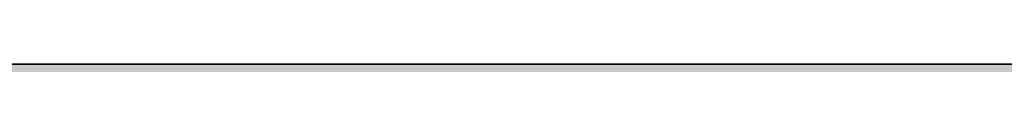
# Model space of a CAD drawing. Units: inches. Extents: x 2091 to 2899, y 967 to 2217.
# Tile 94 of 256: x 2251.3854 to 2251.5278, y 1099.9191 to 1099.9191. Entities that reach past the tile are written whole.
import ezdxf

# ---------------------------------------------------------------- set-up
doc = ezdxf.new("R2010")
doc.units = ezdxf.units.IN
doc.layers.add('A-WALL-PATT', color=141, linetype='Continuous', lineweight=13, true_color=0xadddf7)
doc.layers.add('L-SITE-WALL', color=7, linetype='Continuous', lineweight=35)

msp = doc.modelspace()

# ---------------------------------------------------------------- hatches: boundary and pattern name
at = {"layer": 'A-WALL-PATT'}
h = msp.add_hatch(color=256, dxfattribs=at)
h.dxf.hatch_style = 1
h.paths.add_polyline_path([(2212.1436, 1941.41906), (2387.6436, 1941.41906), (2387.6436, 1824.41906), (2392.1436, 1824.41906), (2392.1436, 1941.41906), (2609.6436, 1941.41906), (2609.6436, 1825.91906), (2614.1436, 1825.91906), (2614.1436, 1941.41906), (2794.1436, 1941.41906), (2794.1436, 1928.76217), (2803.1436, 1928.76217), (2803.1436, 2050.91906), (2203.1436, 2050.91906), (2203.1436, 1900.75786), (2212.1436, 1900.75786)])
h.paths.add_polyline_path([(2212.1436, 1945.91906), (2212.1436, 2041.91906), (2794.1436, 2041.91906), (2794.1436, 1945.91906), (2402.24824, 1945.91906), (2401.10243, 1945.77583), (2398.70243, 1945.77583)], flags=16)
h.paths.add_polyline_path([(2230.22986, 1948.06279), (2227.34986, 1949.50279), (2225.90986, 1951.90279), (2223.98986, 1952.86279), (2223.02986, 1955.26279), (2222.06986, 1959.58279), (2222.06986, 1963.42279), (2223.02986, 1965.66279), (2223.98986, 1965.34279), (2225.58591, 1963.86075), (2226.91153, 1964.95726), (2226.94886, 1965.93879), (2227.77832, 1966.95214), (2228.19992, 1968.8787), (2230.70986, 1964.86279), (2233.58986, 1966.30279), (2233.60731, 1966.33187), (2233.77266, 1964.9382), (2234.6338, 1963.67647), (2235.02986, 1963.90279), (2236.28203, 1965.57236), (2235.98986, 1962.94279), (2237.95451, 1957.54), (2238.38986, 1957.90279), (2239.21586, 1960.30579), (2238.65457, 1966.38496), (2238.69279, 1966.43807), (2238.84058, 1967.49971), (2238.78029, 1967.68749), (2238.88054, 1967.78676), (2238.66686, 1966.25179), (2239.21586, 1960.30579), (2238.38986, 1957.90279), (2236.94986, 1956.70279), (2234.54986, 1949.98279)], flags=0)
h.paths.add_polyline_path([(2278.01197, 1948.06279), (2276.49643, 1947.87335), (2275.84983, 1947.68861), (2274.65197, 1947.10279)], flags=0)
h.paths.add_polyline_path([(2269.85197, 1955.74279), (2268.27618, 1956.62933), (2270.8673, 1956.3484), (2269.37197, 1958.14279), (2268.71496, 1959.19233), (2270.56983, 1958.72861), (2268.58073, 1961.90609), (2270.81197, 1960.89188), (2270.81197, 1963.42279), (2271.39331, 1964.77926), (2270.29176, 1966.1562), (2271.77197, 1965.66279), (2272.14139, 1966.52476), (2273.92983, 1965.92861), (2275.63039, 1968.0543), (2276.33194, 1966.72186), (2276.52043, 1966.95214), (2276.94203, 1968.8787), (2277.73429, 1967.61108), (2278.13989, 1969.46452), (2279.65912, 1967.03374), (2280.41197, 1966.78279), (2280.9493, 1967.58879), (2281.60983, 1967.36861), (2282.13327, 1968.15376), (2282.34924, 1966.33344), (2282.34985, 1966.33259), (2283.40755, 1968.09542), (2283.71263, 1965.52402), (2284.32022, 1964.63379), (2284.51181, 1964.88924), (2284.23497, 1965.70479), (2284.50047, 1967.31896), (2284.90794, 1965.41742), (2285.39631, 1966.06858), (2285.43283, 1966.29061), (2285.47334, 1966.17128), (2286.35392, 1967.34539), (2286.22201, 1966.15817), (2287.66349, 1968.08015), (2287.71397, 1968.44279), (2288.4816, 1969.01668), (2288.57399, 1968.7289), (2288.91746, 1969.06904), (2288.60683, 1966.83761), (2288.92873, 1963.35131), (2288.93497, 1963.35679), (2288.92973, 1963.34042), (2289.01528, 1962.41387), (2290.11122, 1963.87513), (2290.13283, 1963.94261), (2290.21767, 1964.01706), (2290.11122, 1963.87513), (2289.15583, 1960.89161), (2288.59404, 1959.25723), (2288.57197, 1959.10279), (2289.53197, 1960.54279), (2290.01197, 1962.46279), (2290.19184, 1962.64266), (2289.76983, 1959.68861), (2286.88983, 1957.28861), (2284.48983, 1950.56861), (2283.31466, 1950.04631), (2283.29197, 1949.98279), (2280.29006, 1948.64861), (2281.12983, 1948.64861), (2282.56983, 1948.16861), (2283.20473, 1948.06279), (2278.97197, 1948.06279), (2276.09197, 1949.50279), (2274.65197, 1951.90279), (2272.73197, 1952.86279)], flags=0)
h.paths.add_polyline_path([(2271.15887, 1958.02177), (2272.96983, 1955.84861), (2272.00983, 1960.16861), (2272.00983, 1964.00861), (2272.62443, 1965.44266), (2274.32802, 1963.86075), (2275.65365, 1964.95726), (2275.63774, 1964.53909), (2277.41223, 1966.00689), (2277.03297, 1965.15679), (2276.82992, 1964.9756), (2276.76601, 1963.29501), (2277.44964, 1962.66022), (2279.45197, 1964.86279), (2282.33197, 1966.30279), (2283.52983, 1966.88861), (2283.29451, 1966.77095), (2283.91299, 1963.8847), (2284.89925, 1964.44827), (2284.73197, 1962.94279), (2286.69662, 1957.54), (2287.13197, 1957.90279), (2287.54191, 1959.09539), (2287.7794, 1958.44231), (2285.68274, 1956.6951), (2285.8765, 1959.79534), (2284.73197, 1962.94279), (2284.89925, 1964.44827), (2283.91299, 1963.8847), (2284.22383, 1962.43412), (2283.42436, 1963.60548), (2281.60983, 1962.56861), (2281.12983, 1960.16861), (2282.08983, 1956.32861), (2283.04983, 1952.96861), (2282.56983, 1950.56861), (2280.16983, 1948.64861), (2279.88332, 1948.79187), (2278.97197, 1948.06279), (2278.97197, 1949.02279), (2278.67231, 1949.39737), (2277.28983, 1950.08861), (2275.84983, 1952.48861), (2273.92983, 1953.44861), (2272.48983, 1954.88861), (2271.92165, 1954.88861), (2271.77197, 1955.26279)], flags=0)
h.paths.add_polyline_path([(2311.99415, 1955.74279), (2312.06272, 1955.67422), (2312.0551, 1955.7085)], flags=0)
h.paths.add_polyline_path([(2331.95615, 1963.95179), (2333.39615, 1965.39179), (2331.07715, 1963.35679), (2330.9986, 1963.11152)], flags=0)
h.paths.add_polyline_path([(2310.55415, 1954.30279), (2307.03981, 1956.27994), (2310.7629, 1955.87628), (2312.47415, 1953.82279), (2313.43415, 1951.42279), (2315.35415, 1950.46279), (2316.79415, 1948.06279), (2317.46615, 1947.72679), (2319.36869, 1947.96461), (2317.75415, 1949.98279), (2317.56953, 1950.61048), (2316.79415, 1951.90279), (2314.87415, 1952.86279), (2313.91415, 1955.26279), (2311.51415, 1958.14279), (2309.37549, 1961.55917), (2311.51415, 1960.33708), (2311.51415, 1961.98279), (2310.60467, 1963.11963), (2311.72661, 1962.47853), (2312.41833, 1964.09256), (2312.25596, 1964.29552), (2313.19415, 1963.98279), (2313.91415, 1965.66279), (2314.64678, 1965.41858), (2315.35415, 1966.30279), (2316.79415, 1967.74279), (2316.15744, 1966.9469), (2317.03411, 1965.28186), (2317.2226, 1965.51214), (2317.77705, 1968.04577), (2318.47411, 1966.72186), (2318.6626, 1966.95214), (2319.0842, 1968.8787), (2321.20705, 1965.48215), (2322.16142, 1966.9137), (2322.55415, 1966.78279), (2322.78599, 1967.13056), (2322.88165, 1966.32429), (2323.31204, 1965.72174), (2323.65129, 1965.89136), (2324.3965, 1967.13338), (2324.65694, 1964.9382), (2324.97199, 1964.47661), (2325.38728, 1967.0015), (2325.94081, 1964.41835), (2327.22893, 1966.13584), (2327.16632, 1965.57236), (2328.05914, 1966.76278), (2328.22458, 1966.24749), (2329.66797, 1967.67691), (2329.66458, 1967.68749), (2329.76482, 1967.78676), (2329.55115, 1966.25179), (2330.10015, 1960.30579), (2329.33281, 1958.07347), (2329.31306, 1957.93523), (2329.63415, 1958.20279), (2330.23415, 1959.10279), (2330.71415, 1961.02279), (2331.03415, 1961.34279), (2330.71415, 1959.10279), (2329.63415, 1958.20279), (2329.27415, 1957.66279), (2327.71211, 1956.3611), (2325.43415, 1949.98279), (2324.33377, 1949.49374), (2323.99415, 1948.54279), (2319.67415, 1946.62279), (2316.79415, 1948.06279), (2315.35415, 1950.46279), (2313.43415, 1951.42279)], flags=0)
h.paths.add_polyline_path([(2321.33568, 1947.95202), (2321.11415, 1948.06279), (2321.11415, 1949.02279), (2319.19415, 1951.42279), (2316.79415, 1959.58279), (2316.66324, 1959.58279), (2315.35415, 1958.14279), (2314.39415, 1958.14279), (2313.1483, 1958.70908), (2312.95415, 1959.58279), (2312.95415, 1960.89188), (2315.83415, 1959.58279), (2316.66324, 1959.58279), (2317.31471, 1960.29941), (2315.0302, 1962.42075), (2316.35582, 1963.51726), (2316.37234, 1963.95162), (2316.4702, 1963.86075), (2317.79582, 1964.95726), (2317.75522, 1963.88969), (2319.17515, 1965.15679), (2319.49841, 1965.88137), (2321.11415, 1965.34279), (2323.23589, 1962.37236), (2325.68635, 1963.77262), (2325.54279, 1962.48058), (2325.19878, 1963.49401), (2324.47851, 1963.08243), (2324.92601, 1960.99412), (2324.07809, 1962.23647), (2322.41479, 1961.28602), (2322.07415, 1959.58279), (2323.03415, 1955.74279), (2323.99415, 1952.38279), (2323.51415, 1949.98279), (2322.14272, 1948.88565), (2322.07415, 1948.54279)], flags=0)
h.paths.add_polyline_path([(2320.20748, 1963.33746), (2320.15415, 1963.42279), (2320.39415, 1963.54279)], flags=0)
h.paths.add_polyline_path([(2353.85053, 1965.8105), (2354.03053, 1965.7505), (2354.33053, 1966.4505), (2354.33053, 1966.9305)], flags=0)
h.paths.add_polyline_path([(2359.02058, 1969.02641), (2359.09838, 1968.90193), (2359.23353, 1969.5195), (2359.23353, 1969.9995)], flags=0)
h.paths.add_polyline_path([(2358.25669, 1966.68167), (2357.9836, 1966.34803), (2358.21127, 1966.14617), (2358.41049, 1966.38957)], flags=0)
h.paths.add_polyline_path([(2357.76847, 1966.05878), (2357.7322, 1965.10497), (2357.75105, 1965.12056), (2357.76953, 1965.6065), (2357.76953, 1966.05784)], flags=0)
h.paths.add_polyline_path([(2359.11153, 1965.3045), (2359.11153, 1964.8245), (2359.84453, 1966.4675), (2359.84453, 1966.9475)], flags=0)
h.paths.add_polyline_path([(2360.22368, 1966.62145), (2360.69853, 1969.3625), (2360.69853, 1969.8425), (2360.21053, 1967.0255), (2360.21053, 1966.6425)], flags=0)
h.paths.add_polyline_path([(2363.45053, 1967.8905), (2363.45053, 1968.3705), (2362.49053, 1966.9305), (2362.65604, 1966.69878)], flags=0)
h.paths.add_polyline_path([(2364.47552, 1966.07883), (2365.85053, 1968.3705), (2365.85053, 1968.8505), (2364.42798, 1966.47958)], flags=0)
h.paths.add_polyline_path([(2366.31353, 1965.8525), (2366.36671, 1965.69583), (2366.80253, 1968.3455), (2366.80253, 1968.8255)], flags=0)
h.paths.add_polyline_path([(2367.16531, 1965.80354), (2367.29053, 1966.9305), (2367.29053, 1967.4105), (2367.1027, 1965.72007)], flags=0)
h.paths.add_polyline_path([(2370.03653, 1959.9735), (2371.01353, 1963.0245), (2371.01353, 1963.5045), (2370.03653, 1960.4535)], flags=0)
h.paths.add_polyline_path([(2371.61053, 1960.2105), (2372.57053, 1961.6505), (2372.57053, 1962.1305), (2371.80253, 1960.9785)], flags=0)
h.paths.add_polyline_path([(2350.87367, 1956.00509), (2351.93053, 1955.8905), (2354.49053, 1953.3305), (2353.85053, 1954.9305), (2351.45053, 1957.8105), (2347.93553, 1963.4255), (2347.93553, 1963.9055), (2351.45053, 1958.2905), (2353.70507, 1955.58505), (2352.89053, 1959.2505), (2352.89053, 1959.7305), (2352.89053, 1961.92479), (2356.73053, 1959.7305), (2358.45447, 1961.62684), (2354.81053, 1965.0105), (2355.03086, 1965.28591), (2358.69109, 1961.88712), (2361.53053, 1965.0105), (2364.3765, 1966.43348), (2364.52439, 1965.18691), (2365.45447, 1963.82418), (2365.88107, 1964.06795), (2365.37053, 1966.4505), (2365.37053, 1966.9305), (2366.81053, 1960.2105), (2366.81053, 1959.7305), (2366.38871, 1952.98141), (2367.77053, 1956.8505), (2368.64123, 1957.57608), (2366.81053, 1962.6105), (2366.81053, 1963.0905), (2368.77518, 1957.68771), (2369.21053, 1958.0505), (2370.00159, 1960.35187), (2369.47523, 1966.05267), (2369.51346, 1966.10578), (2369.51417, 1966.11091), (2369.47523, 1966.53267), (2369.51346, 1966.58578), (2369.61463, 1967.31259), (2369.18253, 1968.6585), (2369.18253, 1969.1385), (2369.60096, 1967.83519), (2369.7012, 1967.93447), (2369.71795, 1968.05474), (2370.14518, 1968.37414), (2369.77871, 1968.01122), (2369.7012, 1967.45447), (2370.46816, 1968.214), (2369.67494, 1967.26577), (2369.51417, 1966.11091), (2370.03653, 1960.4535), (2370.03653, 1959.9735), (2369.44176, 1958.24319), (2370.65053, 1959.2505), (2371.04582, 1962.01756), (2371.13053, 1962.1305), (2370.65053, 1958.7705), (2367.77053, 1956.3705), (2365.37053, 1949.6505), (2362.0791, 1948.18764), (2363.45053, 1947.7305), (2361.05053, 1947.7305), (2360.09053, 1947.7305), (2357.10386, 1947.35717), (2360.09053, 1948.2105), (2358.17053, 1949.1705), (2356.73053, 1951.5705), (2354.81053, 1952.5305), (2351.93053, 1955.4105)], flags=0)
h.paths.add_polyline_path([(2361.05053, 1948.6905), (2359.13053, 1951.0905), (2356.73053, 1959.2505), (2355.77053, 1959.2505), (2352.89053, 1960.55959), (2352.89053, 1961.44479), (2355.89053, 1959.7305), (2356.73053, 1959.7305), (2356.83719, 1959.36783), (2361.53053, 1964.5305), (2363.24842, 1965.38945), (2364.92531, 1963.0418), (2362.49053, 1961.6505), (2362.06386, 1959.51717), (2362.97053, 1955.8905), (2363.93053, 1952.5305), (2363.93053, 1952.0505), (2363.45053, 1949.6505), (2361.05053, 1947.7305)], flags=0)
h.paths.add_polyline_path([(2359.13053, 1951.5705), (2359.29053, 1951.3705), (2361.05053, 1954.4505), (2361.05053, 1954.9305)], flags=0)
h.paths.add_polyline_path([(2357.21953, 1966.5455), (2356.79253, 1968.8145), (2356.79253, 1969.2945), (2357.21953, 1967.0255)], flags=0)
h.paths.add_polyline_path([(2361.05053, 1954.4505), (2361.53053, 1958.7705), (2361.53053, 1959.2505), (2361.05053, 1954.9305)], flags=0)
h.paths.add_polyline_path([(2402.54829, 1948.48608), (2402.30243, 1948.41583), (2402.59043, 1948.41583)], flags=0)
h.paths.add_polyline_path([(2394.14243, 1956.09583), (2395.68505, 1954.55321), (2396.7205, 1953.97068), (2396.06243, 1955.61583), (2395.24138, 1956.6011), (2395.8789, 1956.44171), (2395.10243, 1959.93583), (2395.10243, 1963.77583), (2396.06243, 1966.01583), (2397.02243, 1965.69583), (2398.61848, 1964.21379), (2399.94411, 1965.3103), (2399.98143, 1966.29183), (2400.81089, 1967.30518), (2401.23249, 1969.23174), (2403.53795, 1965.54301), (2403.94198, 1967.38932), (2404.70243, 1967.13583), (2405.46033, 1966.07478), (2406.62243, 1966.65583), (2406.63988, 1966.68491), (2406.80523, 1965.29124), (2406.92569, 1965.11475), (2407.34243, 1964.97583), (2407.87433, 1965.77367), (2408.1691, 1964.39805), (2409.31461, 1965.9254), (2409.21746, 1965.05105), (2409.44523, 1963.13124), (2410.30637, 1961.86951), (2410.70243, 1962.09583), (2411.44227, 1963.08228), (2411.16543, 1963.89783), (2411.61643, 1966.63976), (2411.72536, 1966.79111), (2411.87315, 1967.85275), (2411.81286, 1968.04053), (2411.91311, 1968.1398), (2411.69943, 1966.60483), (2412.24843, 1960.65883), (2413.22543, 1963.70983), (2414.3779, 1964.72116), (2414.51315, 1965.69275), (2414.45286, 1965.88053), (2414.55311, 1965.9798), (2414.3779, 1964.72116), (2414.51982, 1964.8457), (2414.36536, 1964.63111), (2414.33943, 1964.44483), (2414.88843, 1958.49883), (2414.06243, 1956.09583), (2412.62243, 1954.89583), (2410.17137, 1948.03285), (2410.01672, 1948.0844), (2405.90243, 1946.25583), (2405.90243, 1947.21583), (2405.20425, 1948.08856), (2404.22243, 1948.41583), (2403.26243, 1948.41583), (2400.38243, 1949.85583), (2399.66243, 1951.05583), (2397.98243, 1952.73583), (2397.02243, 1953.21583), (2395.68505, 1954.55321), (2392.65678, 1956.25691)], flags=0)
h.paths.add_polyline_path([(2409.08565, 1964.40744), (2409.13036, 1964.27572), (2409.26243, 1964.49583)], flags=0)
h.paths.add_polyline_path([(2397.74243, 1961.61583), (2398.70243, 1963.85583), (2399.66243, 1963.53583), (2401.42656, 1965.74099), (2401.79142, 1966.5588), (2402.07143, 1965.07083), (2402.83551, 1964.39337), (2403.2624, 1964.9149), (2403.33812, 1964.77109), (2402.61552, 1963.97622), (2402.49861, 1960.90224), (2403.543, 1959.93245), (2404.4132, 1960.88968), (2404.70243, 1962.33583), (2407.91635, 1964.17235), (2409.52021, 1961.92694), (2410.98708, 1957.89304), (2411.42243, 1958.25583), (2412.04796, 1960.07562), (2412.41034, 1959.07909), (2411.67562, 1958.46682), (2411.66243, 1958.25583), (2411.62607, 1958.42553), (2409.98243, 1957.05583), (2407.58243, 1950.33583), (2403.26243, 1948.41583), (2403.26243, 1949.37583), (2401.34243, 1951.77583), (2399.41651, 1958.32398), (2397.74243, 1959.08492), (2397.74243, 1959.97012), (2397.10243, 1960.33583), (2397.74243, 1960.04492)], flags=0)
h.paths.add_polyline_path([(2405.90243, 1952.97583), (2405.95043, 1953.40783), (2406.01672, 1953.17583)], flags=0)
h.paths.add_polyline_path([(2449.81778, 1967.11401), (2449.75232, 1967.13583), (2449.7937, 1967.0779)], flags=0)
h.paths.add_polyline_path([(2451.6977, 1966.61812), (2451.74089, 1966.69012), (2451.69205, 1966.6657)], flags=0)
h.paths.add_polyline_path([(2454.34363, 1965.73757), (2455.75232, 1967.61583), (2455.99232, 1968.09583), (2454.3645, 1965.9254)], flags=0)
h.paths.add_polyline_path([(2457.54732, 1968.86383), (2457.78732, 1969.34383), (2457.05432, 1968.79583), (2457.00762, 1968.46034)], flags=0)
h.paths.add_polyline_path([(2456.92178, 1967.85666), (2456.80224, 1968.22902), (2456.723, 1967.6598)], flags=0)
h.paths.add_polyline_path([(2457.30232, 1967.37683), (2457.54232, 1967.85683), (2456.81032, 1966.83983), (2456.74052, 1966.70022), (2456.74902, 1966.60811)], flags=0)
h.paths.add_polyline_path([(2458.27532, 1963.70983), (2458.15534, 1963.33515), (2460.35432, 1965.26483), (2460.59432, 1965.74483)], flags=0)
h.paths.add_polyline_path([(2458.39232, 1962.81583), (2458.36409, 1962.61819), (2459.59232, 1964.25583), (2459.83232, 1964.73583)], flags=0)
h.paths.add_polyline_path([(2459.35232, 1962.81583), (2459.27232, 1962.49583), (2460.07232, 1963.29583), (2460.31232, 1963.77583)], flags=0)
h.paths.add_polyline_path([(2458.68032, 1960.60783), (2458.63232, 1960.41583), (2459.59232, 1961.85583), (2459.83232, 1962.33583)], flags=0)
h.paths.add_polyline_path([(2437.83817, 1956.24265), (2439.19232, 1956.09583), (2441.35232, 1953.93583), (2440.87232, 1955.13583), (2438.47232, 1958.01583), (2438.07156, 1958.65602), (2438.71232, 1958.49583), (2440.6396, 1956.18311), (2439.91232, 1959.45583), (2439.91232, 1963.29583), (2441.35232, 1966.65583), (2441.59232, 1967.13583), (2441.11232, 1966.01583), (2442.07232, 1965.69583), (2443.98899, 1968.09167), (2444.24132, 1966.75083), (2444.9168, 1966.15192), (2445.67657, 1967.08014), (2446.25532, 1969.72483), (2446.49532, 1970.20483), (2446.28238, 1969.23174), (2447.36267, 1967.50327), (2447.72032, 1969.56783), (2447.96032, 1970.04783), (2447.48548, 1967.30678), (2448.79232, 1965.21583), (2448.47232, 1964.86383), (2448.55232, 1964.73583), (2451.45205, 1966.1857), (2451.61512, 1964.81124), (2452.30792, 1963.79617), (2453.23451, 1964.32565), (2454.07232, 1960.41583), (2453.62869, 1953.31765), (2454.79232, 1956.57583), (2455.03232, 1957.05583), (2455.71884, 1957.62793), (2453.83232, 1962.81583), (2453.94097, 1963.79362), (2453.33532, 1965.57783), (2453.82432, 1968.55083), (2454.06432, 1969.03083), (2453.57532, 1966.05783), (2454.04033, 1964.68792), (2453.83232, 1962.81583), (2455.71884, 1957.62793), (2456.36721, 1958.16824), (2457.05832, 1960.17883), (2457.29832, 1960.65883), (2456.47232, 1958.25583), (2457.71773, 1959.29367), (2457.67232, 1958.97583), (2454.88995, 1956.65719), (2453.61414, 1953.08492), (2453.59232, 1952.73583), (2453.35232, 1952.25583), (2453.3596, 1952.3722), (2452.63232, 1950.33583), (2452.39232, 1949.85583), (2449.20375, 1948.43869), (2450.71232, 1947.93583), (2448.07232, 1947.93583), (2447.11232, 1947.93583), (2444.55232, 1947.61583), (2447.1996, 1948.3722), (2445.19232, 1949.37583), (2443.75232, 1951.77583), (2441.83232, 1952.73583), (2438.95232, 1955.61583)], flags=0)
h.paths.add_polyline_path([(2443.99232, 1959.93583), (2444.04032, 1959.77263), (2444.12155, 1959.86199)], flags=0)
h.paths.add_polyline_path([(2442.91232, 1959.93583), (2443.03232, 1959.93583), (2442.44566, 1960.2025)], flags=0)
h.paths.add_polyline_path([(2444.98294, 1965.01968), (2445.27932, 1965.26483), (2445.51932, 1965.74483), (2444.994, 1965.3103)], flags=0)
h.paths.add_polyline_path([(2446.13332, 1965.02983), (2446.33037, 1965.4715), (2444.97032, 1964.25783), (2444.73032, 1963.77783)], flags=0)
h.paths.add_polyline_path([(2442.79232, 1959.45583), (2443.75232, 1959.45583), (2446.15232, 1951.29583), (2446.41232, 1951.75083), (2446.39232, 1951.77583), (2448.0806, 1954.73032), (2448.55232, 1958.97583), (2441.83232, 1965.21583), (2442.15495, 1965.61911), (2448.79232, 1959.45583), (2448.31232, 1955.13583), (2448.07232, 1954.65583), (2446.41232, 1951.75083), (2448.31232, 1949.37583), (2448.31232, 1948.41583), (2450.54089, 1950.19869), (2450.95232, 1952.25583), (2449.99232, 1955.61583), (2449.03232, 1959.45583), (2449.51232, 1961.85583), (2449.75232, 1962.33583), (2449.6749, 1961.94874), (2452.99451, 1963.84565), (2453.06441, 1963.51941), (2452.88461, 1963.78285), (2449.6749, 1961.94874), (2449.27232, 1959.93583), (2450.23232, 1956.09583), (2451.19232, 1952.73583), (2450.71232, 1950.33583), (2450.47232, 1949.85583), (2448.07232, 1947.93583), (2448.07232, 1948.53583), (2445.43232, 1949.85583), (2443.99232, 1952.25583), (2442.07232, 1953.21583), (2441.11232, 1955.61583), (2440.15232, 1959.93583), (2440.15232, 1960.65583)], flags=0)
h.paths.add_polyline_path([(2456.69232, 1966.98583), (2457.60832, 1968.08083), (2457.84832, 1968.56083), (2456.93232, 1967.46583)], flags=0)
h.paths.add_polyline_path([(2489.89657, 1966.58024), (2489.94295, 1966.18935), (2490.74749, 1967.53025), (2491.31912, 1968.95116)], flags=0)
h.paths.add_polyline_path([(2473.56247, 1956.40713), (2477.13998, 1956.01926), (2476.95533, 1956.24083), (2475.10805, 1957.28011), (2476.34749, 1956.97025), (2475.1869, 1958.82422), (2476.91912, 1958.39116), (2475.41164, 1960.79927), (2477.78749, 1959.71934), (2477.78749, 1962.25025), (2477.6374, 1962.43786), (2477.82255, 1962.33206), (2478.35912, 1963.58406), (2478.35912, 1963.67116), (2477.32435, 1964.96463), (2478.71483, 1964.50114), (2479.31912, 1965.91116), (2480.27912, 1965.59116), (2481.78397, 1967.47221), (2482.11649, 1965.70525), (2482.88056, 1965.02778), (2483.20931, 1965.42941), (2483.22017, 1965.71509), (2483.07594, 1965.98902), (2483.71176, 1966.76581), (2484.13049, 1968.67925), (2484.70212, 1970.10016), (2484.48918, 1969.12707), (2486.5029, 1965.90511), (2487.38749, 1965.61025), (2488.15342, 1966.75914), (2488.71702, 1965.97011), (2489.20009, 1966.21164), (2489.33067, 1965.11099), (2490.3939, 1963.62246), (2490.66077, 1963.77496), (2490.49391, 1964.55364), (2490.92306, 1963.92484), (2491.31912, 1964.15116), (2491.33339, 1964.17018), (2491.21049, 1964.53225), (2491.28176, 1964.96554), (2491.42579, 1964.29338), (2494.07648, 1967.82763), (2494.49792, 1966.51494), (2494.59817, 1966.61422), (2494.68949, 1967.27025), (2495.10675, 1967.5822), (2495.12984, 1967.74807), (2495.06955, 1967.93585), (2495.1698, 1968.03513), (2495.03178, 1967.04363), (2495.75382, 1967.75868), (2494.98205, 1966.68644), (2494.95612, 1966.50016), (2495.47902, 1960.83685), (2495.91049, 1962.18425), (2496.48212, 1963.60516), (2496.07269, 1962.32659), (2496.7689, 1962.93754), (2496.59912, 1962.71116), (2496.11912, 1959.35116), (2496.73287, 1960.27179), (2496.98749, 1961.29025), (2497.55912, 1962.71116), (2497.07912, 1960.79116), (2496.50749, 1959.37025), (2495.54749, 1957.93025), (2492.75884, 1955.60638), (2490.83912, 1950.23116), (2490.26749, 1948.81025), (2485.94749, 1946.89025), (2483.06749, 1948.33025), (2481.62749, 1950.73025), (2479.70749, 1951.69025), (2476.82749, 1954.57025)], flags=0)
h.paths.add_polyline_path([(2485.57697, 1948.31339), (2485.55912, 1948.31116), (2485.57876, 1948.31116)], flags=0)
h.paths.add_polyline_path([(2478.64506, 1954.55116), (2478.10904, 1956.96326), (2479.31912, 1955.51116), (2480.27912, 1953.11116), (2482.19912, 1952.15116), (2483.63912, 1949.75116), (2486.51912, 1948.31116), (2486.51912, 1949.27116), (2484.73931, 1951.49593), (2484.02749, 1950.25025), (2481.62749, 1958.41025), (2482.37515, 1959.23267), (2482.19912, 1959.83116), (2483.19757, 1960.92946), (2479.70749, 1964.17025), (2480.60336, 1965.29008), (2481.87517, 1964.10911), (2482.66639, 1964.76358), (2482.61536, 1963.4218), (2482.9892, 1963.07466), (2484.00849, 1963.98425), (2484.68361, 1965.49751), (2484.58012, 1965.40516), (2485.35727, 1967.14711), (2485.12065, 1965.7812), (2486.42749, 1963.69025), (2488.14538, 1964.5492), (2489.82227, 1962.20155), (2490.74749, 1962.73025), (2491.99966, 1964.39981), (2492.07605, 1965.08726), (2492.21289, 1964.68412), (2492.48537, 1965.04743), (2492.27912, 1963.19116), (2494.24377, 1957.78837), (2494.5625, 1958.05398), (2494.93349, 1959.13325), (2495.50512, 1960.55416), (2494.67912, 1958.15116), (2494.10749, 1956.73025), (2494.5625, 1958.05398), (2493.40854, 1957.09235), (2491.70749, 1961.77025), (2491.99966, 1964.39981), (2490.74749, 1962.73025), (2487.71203, 1960.9957), (2487.47912, 1959.83116), (2488.43912, 1955.99116), (2489.39912, 1952.63116), (2488.91912, 1950.23116), (2488.57692, 1949.9574), (2488.34749, 1948.81025), (2487.65172, 1948.25363), (2487.47912, 1948.31116), (2486.51912, 1948.31116), (2483.63912, 1949.75116), (2482.19912, 1952.15116), (2480.27912, 1953.11116), (2478.83912, 1954.55116)], flags=0)
h.paths.add_polyline_path([(2526.64825, 1966.98752), (2526.51734, 1967.03116), (2526.6001, 1966.9153)], flags=0)
h.paths.add_polyline_path([(2528.47064, 1966.44666), (2528.57449, 1966.61973), (2528.45707, 1966.56102)], flags=0)
h.paths.add_polyline_path([(2534.13334, 1967.49616), (2534.15669, 1967.54285), (2534.05984, 1967.4083)], flags=0)
h.paths.add_polyline_path([(2536.16192, 1964.0506), (2535.15734, 1962.71116), (2535.10087, 1962.31587), (2536.11734, 1963.67116), (2536.42053, 1964.27754)], flags=0)
h.paths.add_polyline_path([(2535.15734, 1959.83116), (2536.11734, 1961.27116), (2536.59734, 1962.23116), (2535.25334, 1960.21516)], flags=0)
h.paths.add_polyline_path([(2513.24904, 1956.2848), (2516.22118, 1955.96256), (2514.99734, 1957.43116), (2514.19582, 1958.71154), (2515.47734, 1958.39116), (2516.93189, 1956.64571), (2516.43734, 1958.87116), (2516.43734, 1962.71116), (2516.87269, 1963.72697), (2515.34643, 1965.6348), (2517.39734, 1964.95116), (2517.87734, 1966.07116), (2518.35734, 1967.03116), (2517.87734, 1965.91116), (2518.83734, 1965.59116), (2520.48659, 1967.65272), (2520.76634, 1966.16616), (2521.53042, 1965.48869), (2521.78144, 1965.79537), (2521.80091, 1966.30727), (2521.4778, 1966.92094), (2521.24634, 1967.12616), (2521.1777, 1967.49091), (2521.4778, 1966.92094), (2522.01042, 1966.44869), (2522.25739, 1966.75042), (2522.78034, 1969.14016), (2523.26034, 1970.10016), (2523.0474, 1969.12707), (2524.67313, 1966.5259), (2526.03734, 1966.07116), (2526.79524, 1965.01011), (2527.97707, 1965.60102), (2528.14014, 1964.22657), (2528.66459, 1963.45816), (2529.38862, 1963.87189), (2529.32967, 1964.14699), (2529.48128, 1963.92484), (2529.87734, 1964.15116), (2529.98401, 1964.29338), (2529.78905, 1965.20318), (2530.0624, 1964.3979), (2532.80248, 1968.05135), (2533.14777, 1966.97585), (2533.24802, 1967.07513), (2533.33934, 1967.73116), (2533.67285, 1967.98049), (2533.72802, 1968.03513), (2533.51434, 1966.50016), (2534.02472, 1960.9725), (2534.56034, 1962.64516), (2535.04034, 1963.60516), (2534.06334, 1960.55416), (2533.23734, 1958.15116), (2534.28815, 1959.02684), (2534.19734, 1958.39116), (2531.5126, 1956.15387), (2529.39734, 1950.23116), (2528.91734, 1949.27116), (2526.44877, 1948.17402), (2527.47734, 1947.83116), (2530.35734, 1947.35116), (2524.59734, 1947.35116), (2521.71734, 1948.79116), (2520.27734, 1951.19116), (2518.35734, 1952.15116), (2515.47734, 1955.03116)], flags=0)
h.paths.add_polyline_path([(2523.93476, 1967.19031), (2523.61951, 1966.48369), (2523.7705, 1966.24211)], flags=0)
h.paths.add_polyline_path([(2518.83734, 1953.11116), (2517.87734, 1955.51116), (2516.88498, 1959.97678), (2516.91734, 1959.96207), (2516.91734, 1962.02545), (2520.75734, 1959.83116), (2522.02495, 1961.22553), (2518.35734, 1964.63116), (2519.00259, 1965.43772), (2520.43339, 1964.10911), (2521.30112, 1964.82687), (2521.24516, 1963.35533), (2525.63831, 1959.27598), (2526.03734, 1961.27116), (2529.39734, 1963.19116), (2530.64952, 1964.86073), (2530.66472, 1964.99755), (2530.69196, 1964.91731), (2531.08778, 1965.44507), (2530.94599, 1964.16894), (2530.69196, 1964.91731), (2529.39734, 1963.19116), (2526.3625, 1961.45697), (2526.03734, 1959.83116), (2526.99734, 1955.99116), (2527.95734, 1952.63116), (2527.47734, 1950.23116), (2527.13449, 1949.95687), (2526.97393, 1949.15409), (2526.69734, 1949.03116), (2524.59734, 1947.35116), (2524.59734, 1948.31116), (2524.27734, 1948.71116), (2522.19734, 1949.75116), (2520.75734, 1952.15116)], flags=0)
h.paths.add_polyline_path([(2520.27734, 1958.87116), (2520.85334, 1959.50476), (2523.15734, 1951.67116), (2524.61389, 1954.22013), (2524.59734, 1954.07116), (2522.67734, 1950.71116)], flags=0)
h.paths.add_polyline_path([(2559.37091, 1966.31116), (2559.39841, 1966.32491), (2559.40194, 1966.3453)], flags=0)
h.paths.add_polyline_path([(2549.77091, 1957.19116), (2552.65091, 1954.31116), (2552.13399, 1955.60347), (2550.61091, 1957.43116), (2547.09591, 1963.04616), (2545.77591, 1965.20616), (2549.29091, 1959.59116), (2551.69091, 1956.71116), (2550.79293, 1960.75206), (2550.73091, 1960.78025), (2550.73091, 1964.87116), (2551.69091, 1967.11116), (2552.65091, 1966.79116), (2554.24696, 1965.30911), (2555.03425, 1965.96034), (2555.58167, 1966.64461), (2555.60991, 1967.38716), (2556.43937, 1968.40051), (2556.86097, 1970.32707), (2559.37091, 1966.31116), (2560.69091, 1964.15116), (2562.40881, 1965.01011), (2561.65091, 1966.07116), (2560.33091, 1968.23116), (2561.7585, 1966.23254), (2562.34721, 1967.11561), (2562.43371, 1966.38657), (2563.1278, 1965.3696), (2563.57091, 1965.59116), (2563.58836, 1965.62024), (2563.36254, 1967.52354), (2563.72249, 1965.84379), (2565.06, 1968.07298), (2564.73286, 1965.12872), (2565.11758, 1963.33338), (2567.44462, 1966.43611), (2567.31561, 1967.83333), (2567.35384, 1967.88644), (2567.50163, 1968.94807), (2567.44134, 1969.13585), (2567.54159, 1969.23513), (2567.32791, 1967.70016), (2567.87691, 1961.75416), (2568.74669, 1964.47033), (2568.63561, 1965.67333), (2568.67384, 1965.72644), (2568.82163, 1966.78807), (2568.76134, 1966.97585), (2568.86159, 1967.07513), (2568.64791, 1965.54016), (2568.72613, 1964.69303), (2568.85391, 1964.80516), (2568.74669, 1964.47033), (2568.81724, 1963.70626), (2568.97091, 1963.91116), (2568.86607, 1963.17731), (2569.19691, 1959.59416), (2568.37091, 1957.19116), (2566.93091, 1955.99116), (2564.62027, 1949.52137), (2564.65091, 1949.51116), (2564.61662, 1949.51116), (2564.53091, 1949.27116), (2560.21091, 1947.35116), (2557.33091, 1948.79116), (2556.0452, 1950.93402), (2556.01091, 1950.95116), (2555.85662, 1951.2083), (2553.97091, 1952.15116), (2551.09091, 1955.03116), (2546.65014, 1957.52951)], flags=0)
h.paths.add_polyline_path([(2567.02579, 1959.33023), (2567.03501, 1959.30489), (2567.05091, 1959.35116)], flags=0)
h.paths.add_polyline_path([(2551.96829, 1962.51837), (2553.01091, 1964.95116), (2553.97091, 1964.63116), (2555.56696, 1963.14911), (2556.89258, 1964.24563), (2556.92991, 1965.22716), (2557.14398, 1965.48869), (2556.42007, 1966.13056), (2556.39142, 1966.10499), (2556.37991, 1966.16616), (2556.42007, 1966.13056), (2556.95191, 1966.60516), (2557.09214, 1966.91948), (2557.57087, 1966.01023), (2557.75937, 1966.24051), (2557.41791, 1964.68016), (2556.89258, 1964.24563), (2556.80709, 1961.99757), (2560.69091, 1958.39116), (2560.63553, 1957.8927), (2560.81091, 1957.19116), (2561.77091, 1953.83116), (2561.29091, 1951.43116), (2559.11042, 1949.68677), (2559.15648, 1949.62919), (2563.02652, 1951.34921), (2562.61091, 1949.27116), (2560.21091, 1947.35116), (2560.21091, 1948.31116), (2559.25091, 1949.51116), (2558.89091, 1949.51116), (2558.89091, 1949.96116), (2558.29091, 1950.71116), (2558.0537, 1951.51767), (2556.97091, 1952.87116), (2555.06788, 1959.34146), (2552.05091, 1961.06545), (2552.05091, 1962.47116)], flags=0)
h.paths.add_polyline_path([(2588.33005, 1958.39116), (2588.61025, 1958.11096), (2588.55336, 1958.36695)], flags=0)
h.paths.add_polyline_path([(2594.74545, 1950.49309), (2593.95753, 1953.17202), (2593.13005, 1954.55116), (2591.21005, 1955.51116), (2590.25005, 1957.91116), (2588.30903, 1960.24038), (2586.17731, 1961.20935), (2587.85005, 1960.79116), (2587.25342, 1961.74425), (2588.44131, 1961.06545), (2588.44131, 1962.65553), (2588.42168, 1962.66535), (2588.44131, 1962.71116), (2586.91404, 1964.62026), (2588.87709, 1963.72796), (2589.29005, 1964.69154), (2589.29005, 1966.07116), (2590.25005, 1968.31116), (2591.21005, 1967.99116), (2592.8061, 1966.50911), (2594.13172, 1967.60563), (2594.16905, 1968.58716), (2594.99851, 1969.60051), (2595.4201, 1971.52707), (2597.93005, 1967.51116), (2600.81005, 1968.95116), (2600.8275, 1968.98024), (2600.99285, 1967.58657), (2601.85399, 1966.32484), (2602.10714, 1966.4695), (2602.23635, 1967.25507), (2602.35672, 1966.69338), (2603.50222, 1968.22073), (2603.21005, 1965.59116), (2605.1747, 1960.18837), (2605.50689, 1960.4652), (2605.02602, 1965.67333), (2605.06425, 1965.72644), (2605.21203, 1966.78807), (2605.15174, 1966.97585), (2605.25199, 1967.07513), (2605.34331, 1967.73116), (2605.9529, 1968.1869), (2605.87475, 1969.03333), (2605.91298, 1969.08644), (2606.06077, 1970.14807), (2606.00048, 1970.33585), (2606.10073, 1970.43513), (2605.88705, 1968.90016), (2606.43605, 1962.95416), (2605.61005, 1960.55116), (2605.99704, 1960.87365), (2606.56431, 1962.64516), (2608.24149, 1964.11694), (2608.01005, 1963.19116), (2607.05005, 1961.75116), (2606.63149, 1961.40236), (2606.20131, 1958.39116), (2603.32131, 1955.99116), (2600.92131, 1949.27116), (2596.60131, 1947.35116), (2593.72131, 1948.79116), (2592.85731, 1950.23116), (2592.65005, 1950.23116)], flags=0)
h.paths.add_polyline_path([(2596.60131, 1947.35116), (2596.60131, 1948.31116), (2594.68131, 1950.71116), (2596.15495, 1953.29003), (2595.53005, 1954.07116), (2593.19923, 1961.99596), (2592.65134, 1962.50471), (2591.78015, 1963.00253), (2593.28299, 1964.24563), (2593.32031, 1965.22716), (2594.14977, 1966.24051), (2594.57137, 1968.16707), (2596.18265, 1965.58902), (2596.95127, 1966.43451), (2598.04131, 1966.07116), (2598.79921, 1965.01011), (2599.96131, 1965.59116), (2599.97876, 1965.62024), (2600.14411, 1964.22657), (2601.00526, 1962.96484), (2601.40131, 1963.19116), (2602.65349, 1964.86073), (2602.36131, 1962.23116), (2603.79275, 1958.29472), (2601.97764, 1953.21243), (2601.94621, 1952.70945), (2599.46876, 1951.60836), (2599.00131, 1949.27116)], flags=0)
h.paths.add_polyline_path([(2597.56131, 1958.87116), (2597.67097, 1959.41942), (2597.59505, 1958.7362)], flags=0)
h.paths.add_polyline_path([(2623.6663, 1961.25438), (2625.51916, 1960.79116), (2624.96554, 1961.67553), (2627.19916, 1960.66025), (2627.19916, 1961.15116), (2626.95916, 1962.23116), (2626.95916, 1963.49116), (2625.58232, 1965.21221), (2626.95916, 1964.42545), (2626.95916, 1965.83116), (2626.86916, 1965.86116), (2627.91916, 1968.31116), (2628.87916, 1967.99116), (2630.47521, 1966.50911), (2631.80084, 1967.60563), (2631.83816, 1968.58716), (2632.66762, 1969.60051), (2633.08922, 1971.52707), (2635.59916, 1967.51116), (2638.47916, 1968.95116), (2638.49661, 1968.98024), (2638.66196, 1967.58657), (2639.17627, 1966.83301), (2639.78022, 1967.83958), (2640.02583, 1966.69338), (2641.17134, 1968.22073), (2640.87916, 1965.59116), (2641.11426, 1964.94463), (2641.41134, 1965.34073), (2641.3081, 1964.41159), (2642.84381, 1960.18837), (2643.27916, 1960.55116), (2644.08474, 1962.89474), (2643.78387, 1966.15333), (2643.80683, 1966.18524), (2643.60068, 1968.41805), (2643.52281, 1968.66058), (2643.72988, 1970.14807), (2643.66959, 1970.33585), (2643.76984, 1970.43513), (2643.55616, 1968.90016), (2643.60068, 1968.41805), (2643.90959, 1967.45585), (2644.00984, 1967.55513), (2643.81174, 1966.13208), (2644.10516, 1962.95416), (2644.23877, 1961.35084), (2644.71916, 1961.75116), (2645.03285, 1962.2217), (2645.32216, 1963.12516), (2646.07642, 1963.78705), (2645.03285, 1962.2217), (2644.34516, 1960.07416), (2643.51916, 1957.67116), (2642.07916, 1956.47116), (2639.71961, 1949.86442), (2639.87553, 1949.83843), (2635.35916, 1947.83116), (2632.47916, 1949.27116), (2631.03916, 1951.67116), (2629.11916, 1952.63116), (2628.15916, 1955.03116), (2625.75916, 1957.91116)], flags=0)
h.paths.add_polyline_path([(2627.81631, 1956.57402), (2627.37371, 1958.56571), (2626.37631, 1959.76259), (2627.19916, 1959.35116), (2627.37371, 1958.56571), (2627.91916, 1957.91116), (2628.87916, 1955.51116), (2630.79916, 1954.55116), (2632.23916, 1952.15116), (2633.31502, 1951.61323), (2631.03916, 1959.35116), (2631.49783, 1959.85569), (2630.79916, 1962.23116), (2631.44987, 1962.94694), (2630.71521, 1963.62911), (2632.04084, 1964.72563), (2632.07816, 1965.70716), (2632.29224, 1965.96869), (2631.70534, 1966.48907), (2633.13644, 1967.76614), (2633.32922, 1968.64707), (2634.67472, 1966.49427), (2635.20847, 1967.08139), (2636.79916, 1966.55116), (2637.6764, 1967.86702), (2638.99395, 1966.02246), (2639.70534, 1966.42898), (2641.11916, 1959.83116), (2640.93007, 1956.80571), (2639.43916, 1952.63116), (2638.22746, 1952.09262), (2637.75916, 1949.75116), (2635.35916, 1947.83116), (2635.35916, 1948.79116), (2633.43916, 1951.19116), (2633.31502, 1951.61323), (2632.23916, 1952.15116), (2630.79916, 1954.55116), (2628.87916, 1955.51116)], flags=0)
h.paths.add_polyline_path([(2637.75916, 1953.83116), (2637.27916, 1955.51116), (2636.31916, 1959.35116), (2636.79916, 1961.75116), (2639.23395, 1963.14246), (2637.55706, 1965.49011), (2638.73889, 1966.08102), (2638.90196, 1964.70657), (2639.7631, 1963.44484), (2636.79916, 1961.75116), (2636.5325, 1960.41783), (2637.03916, 1958.39116), (2637.99916, 1955.03116)], flags=0)
h.paths.add_polyline_path([(2668.56741, 1951.43116), (2667.60741, 1953.83116), (2665.20741, 1956.71116), (2662.2939, 1961.36531), (2665.44741, 1959.59116), (2666.64741, 1958.39116), (2666.64741, 1959.97516), (2666.05832, 1960.68207), (2666.64741, 1960.34545), (2666.64741, 1961.99116), (2666.70009, 1962.11409), (2666.40741, 1963.43116), (2666.40741, 1967.27116), (2667.36741, 1969.51116), (2668.32741, 1969.19116), (2669.92346, 1967.70911), (2671.24908, 1968.80563), (2671.28641, 1969.78716), (2672.11587, 1970.80051), (2672.53746, 1972.72707), (2675.04741, 1968.71116), (2677.92741, 1970.15116), (2677.94486, 1970.18024), (2678.11021, 1968.78657), (2678.97135, 1967.52484), (2679.36741, 1967.75116), (2680.61958, 1969.42073), (2680.32741, 1966.79116), (2682.29206, 1961.38837), (2682.72741, 1961.75116), (2683.35831, 1963.58657), (2683.23211, 1964.95333), (2683.27034, 1965.00644), (2683.39322, 1965.88914), (2683.35997, 1966.24921), (2683.35784, 1966.25585), (2683.35923, 1966.25723), (2682.99211, 1970.23333), (2683.03034, 1970.28644), (2683.17812, 1971.34807), (2683.11784, 1971.53585), (2683.21808, 1971.63513), (2683.00441, 1970.10016), (2683.35923, 1966.25723), (2683.45808, 1966.35513), (2683.39322, 1965.88914), (2683.41391, 1965.66502), (2684.42381, 1966.87227), (2683.55341, 1964.15416), (2683.35831, 1963.58657), (2683.79341, 1958.87416), (2682.96741, 1956.47116), (2681.52741, 1955.27116), (2680.10923, 1951.30025), (2680.08493, 1950.91157), (2679.97685, 1950.92959), (2679.12741, 1948.55116), (2674.80741, 1946.63116), (2671.92741, 1948.07116), (2670.48741, 1950.47116)], flags=0)
h.paths.add_polyline_path([(2671.93568, 1953.22702), (2671.68741, 1953.35116), (2670.24741, 1955.75116), (2668.32741, 1956.71116), (2667.35674, 1959.13783), (2669.52741, 1958.15116), (2670.48741, 1958.15116), (2671.47941, 1959.24236), (2670.6844, 1961.94538), (2668.8896, 1963.61198), (2667.30741, 1964.33116), (2668.56741, 1963.91116), (2668.83094, 1964.24057), (2670.24741, 1963.43116), (2672.42214, 1965.82337), (2672.77746, 1967.44707), (2673.23407, 1966.71649), (2674.41192, 1968.01212), (2673.98056, 1965.52211), (2675.28741, 1963.43116), (2675.55407, 1963.56449), (2675.93241, 1965.45616), (2676.24741, 1965.35116), (2677.0053, 1964.29011), (2678.16741, 1964.87116), (2679.60741, 1967.27116), (2680.32741, 1963.91116), (2680.30655, 1963.57748), (2680.34724, 1963.45761), (2680.85958, 1964.14073), (2680.56741, 1961.51116), (2681.10362, 1960.03657), (2678.88741, 1953.83116), (2677.09248, 1953.03341), (2677.68741, 1950.95116), (2677.20741, 1948.55116), (2674.80741, 1946.63116), (2674.80741, 1947.59116), (2672.88741, 1949.99116)], flags=0)
h.paths.add_polyline_path([(2673.98455, 1951.91116), (2674.56741, 1952.93116), (2674.56741, 1951.91116), (2676.96741, 1953.83116), (2677.44741, 1956.23116), (2676.48741, 1959.59116), (2676.24741, 1960.55116), (2679.72959, 1962.54098), (2680.05927, 1961.00248), (2679.21135, 1962.24484), (2676.24741, 1960.55116), (2676.48741, 1959.59116), (2677.44741, 1956.23116), (2676.96741, 1953.83116), (2674.56741, 1951.91116)], flags=0)
h.paths.add_polyline_path([(2707.47928, 1952.81465), (2706.51928, 1955.21465), (2705.55928, 1959.53465), (2705.55928, 1963.37465), (2706.51928, 1965.61465), (2707.47928, 1965.29465), (2709.07533, 1963.81261), (2710.40096, 1964.90912), (2710.43828, 1965.89065), (2711.26774, 1966.904), (2711.68934, 1968.83056), (2714.19928, 1964.81465), (2717.07928, 1966.25465), (2717.09673, 1966.28373), (2717.26208, 1964.89006), (2718.12322, 1963.62833), (2718.51928, 1963.85465), (2719.77146, 1965.52422), (2719.47928, 1962.89465), (2721.44393, 1957.49186), (2721.87928, 1957.85465), (2722.70528, 1960.25765), (2722.14399, 1966.33682), (2722.18221, 1966.38993), (2722.33, 1967.45157), (2722.26971, 1967.63934), (2722.36996, 1967.73862), (2722.15628, 1966.20365), (2722.70528, 1960.25765), (2721.87928, 1957.85465), (2720.43928, 1956.65465), (2718.03928, 1949.93465), (2713.71928, 1948.01465), (2710.83928, 1949.45465), (2709.39928, 1951.85465)], flags=0)
h.paths.add_polyline_path([(2749.30123, 1952.81465), (2748.34123, 1955.21465), (2747.38123, 1959.53465), (2747.38123, 1963.37465), (2748.34123, 1965.61465), (2749.30123, 1965.29465), (2750.89728, 1963.81261), (2752.2229, 1964.90912), (2752.26023, 1965.89065), (2753.08969, 1966.904), (2753.51129, 1968.83056), (2756.02123, 1964.81465), (2758.90123, 1966.25465), (2758.91868, 1966.28373), (2759.08403, 1964.89006), (2759.94517, 1963.62833), (2760.34123, 1963.85465), (2761.5934, 1965.52422), (2761.30123, 1962.89465), (2763.26588, 1957.49186), (2763.70123, 1957.85465), (2764.52723, 1960.25765), (2763.96594, 1966.33682), (2764.00416, 1966.38993), (2764.15195, 1967.45157), (2764.09166, 1967.63934), (2764.19191, 1967.73862), (2763.97823, 1966.20365), (2764.52723, 1960.25765), (2763.70123, 1957.85465), (2762.26123, 1956.65465), (2759.86123, 1949.93465), (2755.54123, 1948.01465), (2752.66123, 1949.45465), (2751.22123, 1951.85465)], flags=0)
h.paths.add_polyline_path([(2212.1436, 1819.93451), (2203.1436, 1819.93451), (2203.1436, 1739.97955), (2212.1436, 1739.97955), (2212.1436, 1780.91906), (2392.1436, 1780.91906), (2392.1436, 1783.91906), (2212.1436, 1783.91906)])
h.paths.add_polyline_path([(2803.1436, 1847.93882), (2794.1436, 1847.93882), (2794.1436, 1785.41906), (2609.6436, 1785.41906), (2493.87561, 1785.41906), (2493.87561, 1780.91906), (2609.6436, 1780.91906), (2794.1436, 1780.91906), (2794.1436, 1696.91906), (2609.37561, 1696.91906), (2609.37561, 1742.91906), (2604.87561, 1742.91906), (2604.87561, 1644.41906), (2609.37561, 1644.41906), (2609.37561, 1692.41906), (2794.1436, 1692.41906), (2794.1436, 1668.16474), (2803.1436, 1668.16474)])
h.paths.add_polyline_path([(2392.1436, 1740.41906), (2387.6436, 1740.41906), (2387.6436, 1629.41906), (2212.1436, 1629.41906), (2212.1436, 1659.1562), (2203.1436, 1659.1562), (2203.1436, 1494.08944), (2212.1436, 1494.08944), (2212.1436, 1627.91906), (2392.1436, 1627.91906)])
h.paths.add_polyline_path([(2457.87561, 1780.91906), (2453.37561, 1780.91906), (2453.37561, 1644.41906), (2568.87561, 1644.41906), (2568.87561, 1648.91906), (2457.87561, 1648.91906)])
h.paths.add_polyline_path([(2545.1436, 1591.91906), (2540.6436, 1591.91906), (2540.6436, 1567.91906), (2468.6436, 1567.91906), (2468.6436, 1627.91906), (2509.1436, 1627.91906), (2509.1436, 1632.41906), (2464.1436, 1632.41906), (2464.1436, 1563.41906), (2545.1436, 1563.41906)])
h.paths.add_polyline_path([(2268.6436, 1555.91906), (2212.1436, 1555.91906), (2212.1436, 1551.41906), (2268.6436, 1551.41906)], flags=17)
h.paths.add_polyline_path([(2212.1436, 1413.26609), (2203.1436, 1413.26609), (2203.1436, 1233.0704), (2212.1436, 1233.0704)])
h.paths.add_polyline_path([(2267.6436, 1351.91906), (2212.1436, 1351.91906), (2212.1436, 1347.41906), (2267.6436, 1347.41906)], flags=17)
h.paths.add_polyline_path([(2456.6436, 1489.41906), (2452.1436, 1489.41906), (2452.1436, 1351.91906), (2312.6436, 1351.91906), (2312.6436, 1347.41906), (2456.6436, 1347.41906)])
h.paths.add_polyline_path([(2472.37017, 1455.41906), (2467.87017, 1455.41906), (2467.87017, 1347.41906), (2472.37017, 1347.41906)])
h.paths.add_polyline_path([(2794.1436, 1351.91906), (2543.37017, 1351.91906), (2543.37017, 1347.41906), (2794.1436, 1347.41906)], flags=17)
h.paths.add_polyline_path([(2312.6436, 1347.41906), (2308.1436, 1347.41906), (2308.1436, 1302.16179), (2308.34197, 1302.16433), (2308.1436, 1298.16925), (2308.1436, 1275.41906), (2212.1436, 1275.41906), (2212.1436, 1270.91906), (2312.6436, 1270.91906)], flags=17)
h.paths.add_polyline_path([(2212.1436, 1152.24706), (2203.1436, 1152.24706), (2203.1436, 1090.91906), (2803.1436, 1090.91906), (2803.1436, 1392.71355), (2794.1436, 1392.71355), (2794.1436, 1143.41906), (2548.03245, 1143.41906), (2548.03245, 1138.91906), (2794.1436, 1138.91906), (2794.1436, 1099.91906), (2212.1436, 1099.91906)])
h.paths.add_polyline_path([(2471.53245, 1266.32853, 0.031658), (2467.03245, 1269.94579), (2467.03245, 1143.41906), (2471.53245, 1143.41906), (2471.53245, 1148.81906)], flags=17)
h.paths.add_polyline_path([(2803.1436, 1587.34139), (2794.1436, 1587.34139), (2794.1436, 1473.5369), (2803.1436, 1473.5369)])
h.paths.add_polyline_path([(2794.1436, 1536.41906), (2651.1436, 1536.41906), (2651.1436, 1531.91906), (2794.1436, 1531.91906)])
h.paths.add_polyline_path([(2614.1436, 1620.41906), (2609.6436, 1620.41906), (2609.6436, 1536.41906), (2614.1436, 1536.41906)])
h.paths.add_polyline_path([(2271.08273, 1964.31724), (2776.85297, 1964.31724), (2776.85297, 2037.16962), (2271.08273, 2037.16962)], flags=8)
h.paths.add_polyline_path([(2380.64929, 1536.82414), (2461.04081, 1536.82414), (2461.04081, 1554.65259), (2380.64929, 1554.65259)], flags=9)
h.paths.add_polyline_path([(2203.65504, 1608.81531), (2316.11844, 1608.81531), (2316.11844, 1621.91836), (2203.65504, 1621.91836)], flags=24)
h.paths.add_polyline_path([(2212.67726, 1313.5041), (2282.59152, 1313.5041), (2282.59152, 1322.74524), (2212.67726, 1322.74524)], flags=24)
h.paths.add_polyline_path([(2457.11198, 1114.77857), (2558.48158, 1114.77857), (2558.48158, 1142.21968), (2457.11198, 1142.21968)], flags=25)
h.paths.add_polyline_path([(2473.44234, 1273.01007), (2604.64123, 1273.01007), (2604.64123, 1318.34693), (2473.44234, 1318.34693)], flags=25)
h.paths.add_polyline_path([(2638.8763, 1626.97743), (2684.25037, 1627.97674), (2684.03848, 1637.59749), (2638.66442, 1636.59819)], flags=9)
h.paths.add_polyline_path([(2537.59055, 1453.79345), (2628.38955, 1453.79345), (2628.38955, 1475.34481), (2537.59055, 1475.34481)], flags=9)
h.paths.add_polyline_path([(2504.13764, 1714.6324), (2554.64719, 1714.6324), (2554.64719, 1730.23771), (2504.13764, 1730.23771)], flags=25)
h.paths.add_polyline_path([(2487.50118, 1575.65187), (2535.09712, 1575.65187), (2535.09712, 1598.37765), (2487.50118, 1598.37765)], flags=25)
h.paths.add_polyline_path([(2709.0994, 1735.71028), (2740.0166, 1735.71028), (2740.0166, 1749.93764), (2709.0994, 1749.93764)], flags=25)
h.paths.add_polyline_path([(2442.43842, 1792.17166), (2564.72884, 1792.17166), (2564.72884, 1842.00016), (2442.43842, 1842.00016)], flags=9)
h.paths.add_polyline_path([(2655.8158, 1809.64408), (2789.52014, 1806.6938), (2790.08498, 1832.29164), (2656.38064, 1835.24192)], flags=25)
h.paths.add_polyline_path([(2234.8427, 1797.72014), (2368.59285, 1794.76885), (2369.16072, 1820.50413), (2235.41056, 1823.45542)], flags=9)
h.paths.add_polyline_path([(2245.13847, 1644.00633), (2398.42773, 1640.6239), (2398.99484, 1666.32482), (2245.70557, 1669.70725)], flags=9)
h.paths.add_polyline_path([(2306.14285, 1431.16852), (2413.76831, 1428.79369), (2414.33315, 1454.39153), (2306.70768, 1456.76636)], flags=9)
h.paths.add_polyline_path([(2306.83458, 1458.23314), (2393.38048, 1456.32345), (2393.93281, 1481.35436), (2307.38691, 1483.26405)], flags=9)

# ---------------------------------------------------------------- linework, layer by layer
at = {"layer": 'L-SITE-WALL'}
msp.add_line((2794.1436, 1099.91906), (2212.1436, 1099.91906), dxfattribs=at)

doc.saveas('drawing.dxf')
